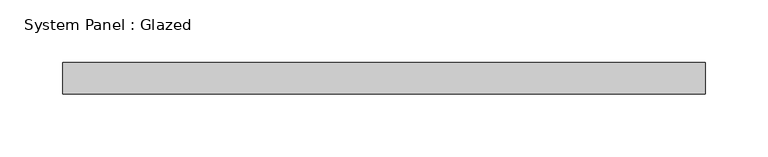
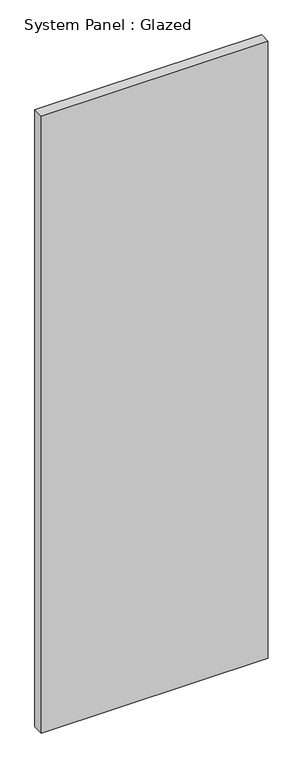
"""IFC4 building model written with IfcOpenShell, lengths in millimetres: plate geometry, System Panel : Glazed."""

from ifc_helpers import new_model, si_unit, origin, origin_with_axes, place, context, project, spatial, polyline, outline, extrude, source, transform, mapped, element, save


def system_panel_glazed_438a3505(model_context):
    return source(origin(), model_context, "Body", "SweptSolid", [
        extrude(outline(polyline([(257.175, 19.05), (-257.175, 19.05), (-257.175, 44.45), (257.175, 44.45), (257.175, 19.05)])), origin_with_axes(), (0.0, 0.0, 1.0), 1480.0454815),
    ])


if __name__ == "__main__":
    model = new_model("IFC4")
    model_context = context("Model", 3, world=origin())
    ifc_project = project(units=[si_unit("LENGTHUNIT", "METRE", prefix="MILLI")], contexts=[model_context])
    site = spatial("IfcSite", under=ifc_project)
    building = spatial("IfcBuilding", under=site)
    placement = place(None, origin())
    system_panel_glazed_shape = system_panel_glazed_438a3505(model_context)
    element("IfcPlate", 1, ObjectType="System Panel : Glazed", at=placement, inside=building, context=model_context, shape_type="MappedRepresentation", body=[
        mapped(system_panel_glazed_shape, transform((0.0, 0.0, 0.0), x_axis=(1.0, 0.0, 0.0), y_axis=(0.0, 1.0, 0.0), z_axis=(0.0, 0.0, 1.0))),
    ])
    save(model, "model.ifc")

# Revit data of these elements
# Type "System Panel : Glazed"
#   Construction Type Id = "GSP4R"
#   Analytic Construction = "1/8 in Pilkington single glazing"
#   Visual Light Transmittance = 0.9
#   Solar Heat Gain Coefficient = 0.86
#   Heat Transfer Coefficient (U) = 1.18115 BTU/(h·ft²·°F)
#   Define Thermal Properties by = 1
# Element 1 (IfcPlate, "System Panel : Glazed")
#   Materials on its faces: "Glass"
# Materials
#   "Glass": class "Glass", colour RGB 0 128 192, transparency 0.75, Description = "Soda Lime Glass", Cost = 0
